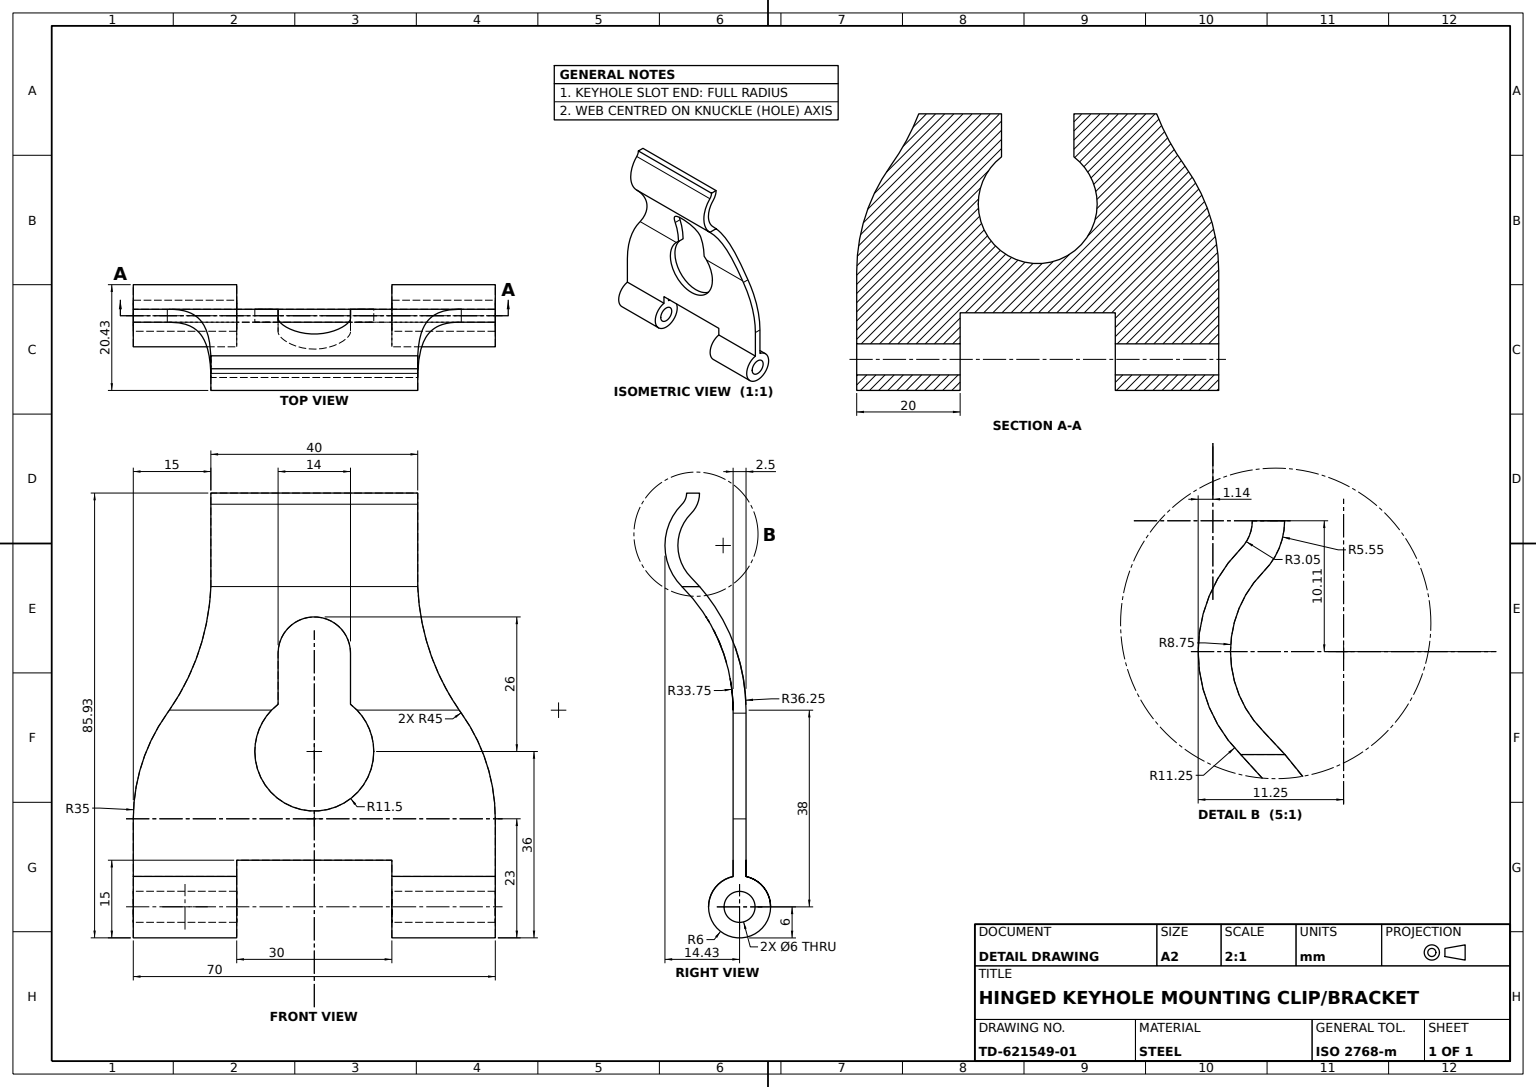
SolidWorks part; units mm, degrees
material "Plain Carbon Steel"
ref_plane "Front Plane" through (0, 0, 0) normal (0, 0, 1) x (1, 0, 0)
ref_plane "Top Plane" through (0, 0, 0) normal (0, 1, 0) x (1, 0, 0)
ref_plane "Right Plane" through (0, 0, 0) normal (1, 0, 0) x (0, 0, -1)
sketch "Bracket Side Profile Sketch" plane through (0, 0, 0) normal (1, 0, 0) x (0, 0, -1)
  line L0 (0, 0) -> (0, 38) construction
  line L1 (1.25, 5.8683) -> (1.25, 38)
  line L2 (-8.9918, 79.9314) -> (-24.4309, 79.9314) construction
  line L3 (-35, 38) -> (-3.1802, 69.8198) construction
  line L5 (-35, 38) -> (35.6486, 38) construction
  line L7 (-3.1802, 69.8198) -> (-21.0764, 87.716) construction
  line L8 (-1.25, 5.8683) -> (-1.25, 38)
  line L9 (-10.2418, 79.9314) -> (-7.7418, 79.9314)
  arc A0 (-1.25, 5.8683) -> (1.25, 5.8683) centre (0, 0) ccw
  circle A1 centre (0, 0) radius 3
  arc A2 (0, 38) -> (-10.2513, 62.7487) centre (-35, 38) ccw construction
  arc A3 (-10.2513, 62.7487) -> (-10.2513, 76.8909) centre (-3.1802, 69.8198) cw construction
  arc A4 (-10.2513, 76.8909) -> (-8.9918, 79.9314) centre (-13.2918, 79.9314) ccw construction
  arc A5 (1.25, 38) -> (-9.3674, 63.6326) centre (-35, 38) ccw
  arc A8 (-1.25, 38) -> (-11.1351, 61.8649) centre (-35, 38) ccw
  arc A9 (-11.1351, 61.8649) -> (-11.1351, 77.7748) centre (-3.1802, 69.8198) cw
  arc A10 (-11.1351, 77.7748) -> (-10.2418, 79.9314) centre (-13.2918, 79.9314) ccw
  arc A11 (-9.3674, 63.6326) -> (-9.3674, 76.007) centre (-3.1802, 69.8198) cw
  arc A12 (-9.3674, 76.007) -> (-7.7418, 79.9314) centre (-13.2918, 79.9314) ccw
  dimension "D1" = 12
  dimension "D2" = 6
  dimension "D5" = 35
  dimension "D6" = 10
  dimension "D8" = 4.3
  dimension "D3" = 38
  dimension "D4" = 2.5
  dimension "D7" = 45
  dimension "D9" = 45
extrude "Bracket Body Extrude 70mm" add sketch "Bracket Side Profile Sketch" along normal mid plane 70
sketch "Outline and Keyhole Sketch" plane through (0, 0, 1.25) normal (0, 0, 1) x (1, 0, 0)
  line L0 (-46.2107, 0) -> (50.4969, 0) construction
  line L1 (35, -6) -> (35, 17)
  line L3 (35, 38) -> (35, 5.8683) construction
  line L4 (35, -6) -> (15, -6)
  line L5 (0, 88.9234) -> (0, -13.9456) construction
  line L6 (35, 61.8649) -> (-35, 61.8649) construction
  line L7 (20, 61.8649) -> (20, 79.9314)
  line L8 (35, 79.9314) -> (-35, 79.9314) construction
  line L9 (-35, -6) -> (35, -6) construction
  line L10 (15, -6) -> (15, 9)
  line L12 (-20, 61.8649) -> (-20, 79.9314)
  line L13 (-35, -6) -> (-35, 17)
  line L14 (-35, -6) -> (-15, -6)
  line L15 (-15, -6) -> (-15, 9)
  line L16 (-15, 9) -> (15, 9)
  line L17 (-20, 79.9314) -> (20, 79.9314)
  line L18 (7, 49) -> (7, 39.1241)
  line L19 (-7, 49) -> (-7, 39.1241)
  arc A0 (35, 17) -> (28.4213, 37.4262) centre (0, 17) ccw
  arc A1 (28.4213, 37.4262) -> (20, 61.8649) centre (64.963, 63.6884) cw
  arc A2 (-28.4213, 37.4262) -> (-20, 61.8649) centre (-64.963, 63.6884) ccw
  arc A3 (-35, 17) -> (-28.4213, 37.4262) centre (0, 17) cw
  arc A4 (-7, 39.1241) -> (7, 39.1241) centre (0, 30) ccw
  arc A5 (7, 49) -> (-7, 49) centre (0, 49) ccw
  dimension "D6" = 45
  dimension "D7" = 35
  dimension "D9" = 23
  dimension "D11" = 7
  dimension "D1" = 30
  dimension "D2" = 15
  dimension "D3" = 15
  dimension "D4" = 40
  dimension "D5" = 17
  dimension "D8" = 30
  dimension "D10" = 19
extrude "Outline and Keyhole Cut" cut sketch "Outline and Keyhole Sketch" against normal through all both and the other way through all flip side to cut
